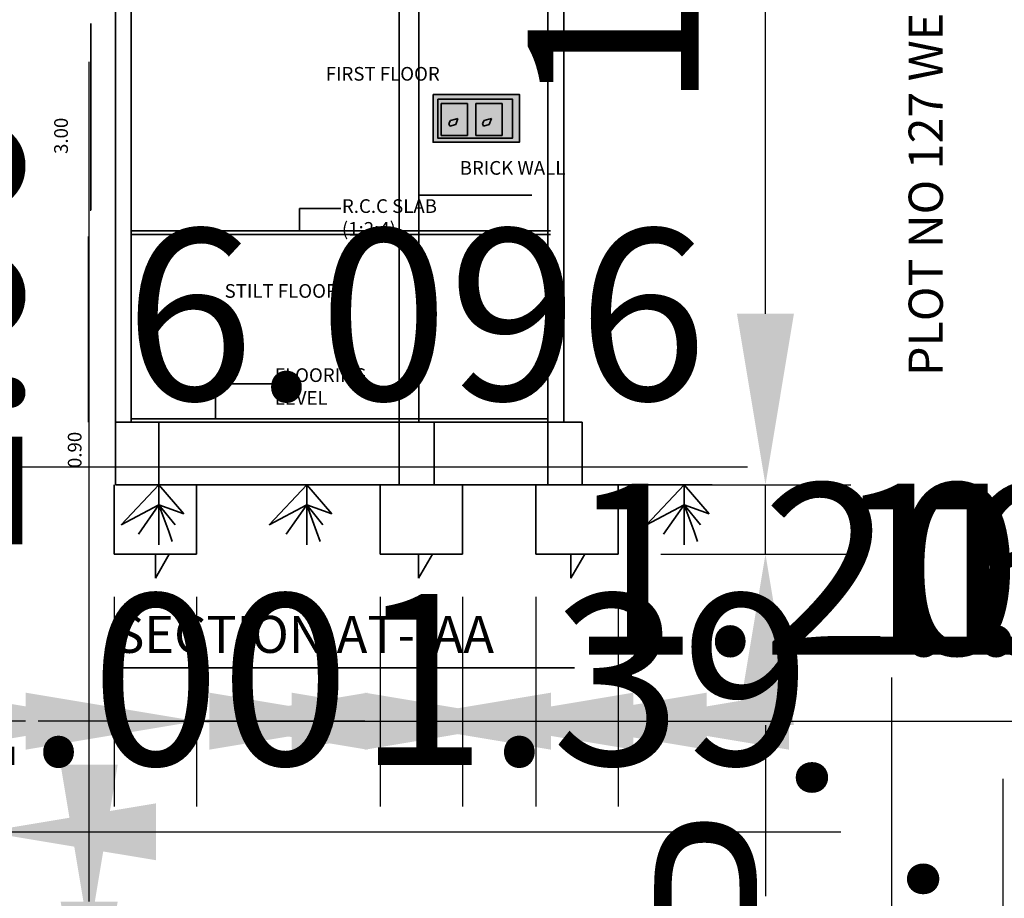
# Model space of a CAD drawing. Units: metres. Extents: x 782 to 1487, y 1262 to 7446.
# Tile 20 of 25: x 801.93 to 816.33, y 1313.5 to 1326.35. Entities that reach past the tile are written whole.
import ezdxf

# ---------------------------------------------------------------- set-up
doc = ezdxf.new("R2010")
doc.units = ezdxf.units.M
for name, color, linetype, lineweight in [('A-ANNO-DIMS', 2, 'Continuous', 18), ('A-ANNO-TEXT', 3, 'Continuous', 18), ('A-SECT', 7, 'Continuous', 35), ('A-SECT-PATT', 9, 'Continuous', 13)]:
    doc.layers.add(name, color=color, linetype=linetype, lineweight=lineweight)
doc.styles.get("Standard").update_dxf_attribs({"font": 'arial.ttf'})
doc.dimstyles.new('ISO-25', dxfattribs={"dimtxt": 2.5, "dimasz": 2.5, "dimexe": 1.25, "dimexo": 0.625, "dimtad": 1, "dimtxsty": 'Standard', "dimcen": 2.5, "dimadec": 0, "dimazin": 0, "dimtfac": 1, "dimtmove": 0, "dimatfit": 3, "dimfxl": 1, "dimarcsym": 0})

# ---------------------------------------------------------------- blocks, each defined once
blk = doc.blocks.new('*D2')
at = {"layer": 'A-ANNO-DIMS', "color": 0, "lineweight": -2, "transparency": 16777216}
for p, q in [((794.559, 1311.575), (794.559, 1314.2)), ((800.039, 1311.575), (800.039, 1314.2)), ((792.059, 1312.95), (781.81, 1312.95)), ((800.039, 1312.95), (794.559, 1312.95)), ((802.539, 1312.95), (805.039, 1312.95))]:
    blk.add_line(p, q, dxfattribs=at)
at = {"layer": 'A-ANNO-DIMS', "color": 0, "transparency": 16777216}
for points in [[(792.059, 1313.367), (792.059, 1312.534), (794.559, 1312.95)], [(802.539, 1313.367), (802.539, 1312.534), (800.039, 1312.95)]]:
    blk.add_solid(points, dxfattribs=at)
at = {"layer": 'Defpoints', "color": 0, "transparency": 16777216}
for p in [(794.559, 1312.95), (794.559, 1310.95), (800.039, 1310.95)]:
    blk.add_point(p, dxfattribs=at)
at = {"layer": 'A-ANNO-DIMS', "color": 0, "transparency": 16777216, "insert": (785.685, 1315.078), "char_height": 2.5, "width": 6.51678, "attachment_point": 5}
blk.add_mtext('5,48', dxfattribs=at)
blk = doc.blocks.new('*D23')
at = {"layer": 'A-ANNO-DIMS', "color": 0, "lineweight": -2, "transparency": 16777216}
for p, q in [((816.313, 1296.414), (816.313, 1315.246)), ((816.313, 1293.067), (816.313, 1293.914)), ((816.804, 1293.914), (817.563, 1293.914)), ((816.804, 1293.067), (817.563, 1293.067)), ((816.313, 1290.567), (816.313, 1288.067))]:
    blk.add_line(p, q, dxfattribs=at)
at = {"layer": 'A-ANNO-DIMS', "color": 0, "transparency": 16777216}
for points in [[(815.896, 1296.414), (816.729, 1296.414), (816.313, 1293.914)], [(815.896, 1290.567), (816.729, 1290.567), (816.313, 1293.067)]]:
    blk.add_solid(points, dxfattribs=at)
at = {"layer": 'Defpoints', "color": 0, "transparency": 16777216}
for p in [(816.179, 1293.914), (816.313, 1293.914), (816.179, 1293.067)]:
    blk.add_point(p, dxfattribs=at)
at = {"layer": 'A-ANNO-DIMS', "color": 0, "transparency": 16777216, "insert": (814.411, 1307.08), "char_height": 2.5, "attachment_point": 5, "rotation": 90}
blk.add_mtext('0.85 TYP.', dxfattribs=at)
blk = doc.blocks.new('*D25')
at = {"layer": 'A-ANNO-DIMS', "color": 0, "lineweight": -2, "transparency": 16777216}
for p, q in [((814.687, 1297.897), (814.687, 1316.729)), ((814.687, 1294.551), (814.687, 1295.397)), ((815.184, 1295.397), (815.937, 1295.397)), ((815.184, 1294.551), (815.937, 1294.551)), ((814.687, 1292.051), (814.687, 1289.551))]:
    blk.add_line(p, q, dxfattribs=at)
at = {"layer": 'A-ANNO-DIMS', "color": 0, "transparency": 16777216}
for points in [[(814.27, 1297.897), (815.103, 1297.897), (814.687, 1295.397)], [(814.27, 1292.051), (815.103, 1292.051), (814.687, 1294.551)]]:
    blk.add_solid(points, dxfattribs=at)
at = {"layer": 'Defpoints', "color": 0, "transparency": 16777216}
for p in [(814.559, 1295.397), (814.687, 1295.397), (814.559, 1294.551)]:
    blk.add_point(p, dxfattribs=at)
at = {"layer": 'A-ANNO-DIMS', "color": 0, "transparency": 16777216, "insert": (812.785, 1308.563), "char_height": 2.5, "attachment_point": 5, "rotation": 90}
blk.add_mtext('0.85 TYP.', dxfattribs=at)
blk = doc.blocks.new('*D37')
at = {"layer": 'A-ANNO-DIMS', "color": 0, "lineweight": -2, "transparency": 16777216}
for p, q in [((802.949, 1313.45), (802.949, 1315.95)), ((800.664, 1310.95), (804.199, 1310.95)), ((802.949, 1310.95), (802.949, 1307.03)), ((800.653, 1307.03), (804.199, 1307.03)), ((802.949, 1304.53), (802.949, 1294.314))]:
    blk.add_line(p, q, dxfattribs=at)
at = {"layer": 'A-ANNO-DIMS', "color": 0, "transparency": 16777216}
for points in [[(802.532, 1313.45), (803.366, 1313.45), (802.949, 1310.95)], [(802.532, 1304.53), (803.366, 1304.53), (802.949, 1307.03)]]:
    blk.add_solid(points, dxfattribs=at)
at = {"layer": 'Defpoints', "color": 0, "transparency": 16777216}
for p in [(800.039, 1310.95), (800.028, 1307.03), (802.949, 1307.03)]:
    blk.add_point(p, dxfattribs=at)
at = {"layer": 'A-ANNO-DIMS', "color": 0, "transparency": 16777216, "insert": (801.047, 1298.172), "char_height": 2.5, "attachment_point": 5, "rotation": 90}
blk.add_mtext('3.92', dxfattribs=at)
blk = doc.blocks.new('*D43')
at = {"layer": 'A-ANNO-DIMS', "color": 0, "lineweight": -2, "transparency": 16777216}
for p, q in [((792.559, 1313.575), (792.559, 1315.72)), ((794.559, 1311.575), (794.559, 1315.72)), ((790.059, 1314.47), (787.559, 1314.47)), ((792.559, 1314.47), (794.559, 1314.47)), ((797.059, 1314.47), (807.337, 1314.47))]:
    blk.add_line(p, q, dxfattribs=at)
at = {"layer": 'A-ANNO-DIMS', "color": 0, "transparency": 16777216}
for points in [[(790.059, 1314.887), (790.059, 1314.054), (792.559, 1314.47)], [(797.059, 1314.887), (797.059, 1314.054), (794.559, 1314.47)]]:
    blk.add_solid(points, dxfattribs=at)
at = {"layer": 'Defpoints', "color": 0, "transparency": 16777216}
for p in [(794.559, 1314.47), (792.559, 1312.95), (794.559, 1310.95)]:
    blk.add_point(p, dxfattribs=at)
at = {"layer": 'A-ANNO-DIMS', "color": 0, "transparency": 16777216, "insert": (803.448, 1316.372), "char_height": 2.5, "attachment_point": 5}
blk.add_mtext('2.00', dxfattribs=at)
blk = doc.blocks.new('*D44')
at = {"layer": 'A-ANNO-DIMS', "color": 0, "lineweight": -2, "transparency": 16777216}
for p, q in [((800.039, 1311.575), (800.039, 1315.72)), ((801.429, 1313.575), (801.429, 1315.72)), ((797.539, 1314.47), (795.039, 1314.47)), ((800.039, 1314.47), (801.429, 1314.47)), ((803.929, 1314.47), (813.943, 1314.47))]:
    blk.add_line(p, q, dxfattribs=at)
at = {"layer": 'A-ANNO-DIMS', "color": 0, "transparency": 16777216}
for points in [[(797.539, 1314.887), (797.539, 1314.054), (800.039, 1314.47)], [(803.929, 1314.887), (803.929, 1314.054), (801.429, 1314.47)]]:
    blk.add_solid(points, dxfattribs=at)
at = {"layer": 'Defpoints', "color": 0, "transparency": 16777216}
for p in [(801.429, 1314.47), (801.429, 1312.95), (800.039, 1310.95)]:
    blk.add_point(p, dxfattribs=at)
at = {"layer": 'A-ANNO-DIMS', "color": 0, "transparency": 16777216, "insert": (810.186, 1316.373), "char_height": 2.5, "attachment_point": 5}
blk.add_mtext('1.39', dxfattribs=at)
blk = doc.blocks.new('*D47')
at = {"layer": 'A-ANNO-DIMS', "color": 0, "lineweight": -2, "transparency": 16777216}
for p, q in [((802.949, 1315.45), (802.949, 1325.728)), ((802.054, 1312.95), (804.199, 1312.95)), ((802.949, 1310.95), (802.949, 1312.95)), ((800.664, 1310.95), (804.199, 1310.95)), ((802.949, 1308.45), (802.949, 1305.95))]:
    blk.add_line(p, q, dxfattribs=at)
at = {"layer": 'A-ANNO-DIMS', "color": 0, "transparency": 16777216}
for points in [[(802.532, 1315.45), (803.366, 1315.45), (802.949, 1312.95)], [(802.532, 1308.45), (803.366, 1308.45), (802.949, 1310.95)]]:
    blk.add_solid(points, dxfattribs=at)
at = {"layer": 'Defpoints', "color": 0, "transparency": 16777216}
for p in [(801.429, 1312.95), (802.949, 1312.95), (800.039, 1310.95)]:
    blk.add_point(p, dxfattribs=at)
at = {"layer": 'A-ANNO-DIMS', "color": 0, "transparency": 16777216, "insert": (801.048, 1321.839), "char_height": 2.5, "attachment_point": 5, "rotation": 90}
blk.add_mtext('2.00', dxfattribs=at)
blk = doc.blocks.new('*D115')
at = {"layer": 'A-ANNO-DIMS', "color": 0, "lineweight": -2, "transparency": 16777216}
for p, q in [((789.282, 1319.809), (786.782, 1319.809)), ((791.782, 1319.834), (791.782, 1318.559)), ((791.782, 1319.809), (797.878, 1319.809)), ((797.878, 1319.834), (797.878, 1318.559)), ((800.378, 1319.809), (812.576, 1319.809))]:
    blk.add_line(p, q, dxfattribs=at)
at = {"layer": 'A-ANNO-DIMS', "color": 0, "transparency": 16777216}
for points in [[(789.282, 1320.226), (789.282, 1319.392), (791.782, 1319.809)], [(800.378, 1320.226), (800.378, 1319.392), (797.878, 1319.809)]]:
    blk.add_solid(points, dxfattribs=at)
at = {"layer": 'Defpoints', "color": 0, "transparency": 16777216}
for p in [(791.782, 1320.459), (797.878, 1320.459), (797.878, 1319.809)]:
    blk.add_point(p, dxfattribs=at)
at = {"layer": 'A-ANNO-DIMS', "color": 0, "transparency": 16777216, "insert": (807.727, 1321.711), "char_height": 2.5, "attachment_point": 5}
blk.add_mtext('6.096', dxfattribs=at)
blk = doc.blocks.new('*D140')
at = {"layer": 'A-ANNO-DIMS', "color": 0, "lineweight": -2, "transparency": 16777216}
for p, q in [((803.316, 1317.905), (803.316, 1314.838)), ((804.52, 1317.905), (804.52, 1314.838)), ((800.816, 1316.088), (798.316, 1316.088)), ((803.316, 1316.088), (804.52, 1316.088)), ((807.02, 1316.088), (817.02, 1316.088))]:
    blk.add_line(p, q, dxfattribs=at)
at = {"layer": 'A-ANNO-DIMS', "color": 0, "transparency": 16777216}
for points in [[(800.816, 1316.505), (800.816, 1315.671), (803.316, 1316.088)], [(807.02, 1316.505), (807.02, 1315.671), (804.52, 1316.088)]]:
    blk.add_solid(points, dxfattribs=at)
at = {"layer": 'Defpoints', "color": 0, "transparency": 16777216}
for p in [(803.316, 1318.53), (804.52, 1318.53), (804.52, 1316.088)]:
    blk.add_point(p, dxfattribs=at)
at = {"layer": 'A-ANNO-DIMS', "color": 0, "transparency": 16777216, "insert": (813.27, 1317.989), "char_height": 2.5, "attachment_point": 5}
blk.add_mtext('1.20', dxfattribs=at)
blk = doc.blocks.new('*D141')
at = {"layer": 'A-ANNO-DIMS', "color": 0, "lineweight": -2, "transparency": 16777216}
for p, q in [((804.52, 1317.905), (804.52, 1314.838)), ((807.205, 1317.905), (807.205, 1314.838)), ((802.02, 1316.088), (799.52, 1316.088)), ((804.52, 1316.088), (807.205, 1316.088)), ((809.705, 1316.088), (819.997, 1316.088))]:
    blk.add_line(p, q, dxfattribs=at)
at = {"layer": 'A-ANNO-DIMS', "color": 0, "transparency": 16777216}
for points in [[(802.02, 1316.505), (802.02, 1315.671), (804.52, 1316.088)], [(809.705, 1316.505), (809.705, 1315.671), (807.205, 1316.088)]]:
    blk.add_solid(points, dxfattribs=at)
at = {"layer": 'Defpoints', "color": 0, "transparency": 16777216}
for p in [(804.52, 1318.53), (807.205, 1318.53), (807.205, 1316.088)]:
    blk.add_point(p, dxfattribs=at)
at = {"layer": 'A-ANNO-DIMS', "color": 0, "transparency": 16777216, "insert": (816.101, 1317.989), "char_height": 2.5, "attachment_point": 5}
blk.add_mtext('2.68', dxfattribs=at)
blk = doc.blocks.new('*D142')
at = {"layer": 'A-ANNO-DIMS', "color": 0, "lineweight": -2, "transparency": 16777216}
for p, q in [((807.205, 1317.905), (807.205, 1314.838)), ((808.409, 1317.905), (808.409, 1314.838)), ((804.705, 1316.088), (802.205, 1316.088)), ((807.205, 1316.088), (808.409, 1316.088)), ((810.909, 1316.088), (820.909, 1316.088))]:
    blk.add_line(p, q, dxfattribs=at)
at = {"layer": 'A-ANNO-DIMS', "color": 0, "transparency": 16777216}
for points in [[(804.705, 1316.505), (804.705, 1315.671), (807.205, 1316.088)], [(810.909, 1316.505), (810.909, 1315.671), (808.409, 1316.088)]]:
    blk.add_solid(points, dxfattribs=at)
at = {"layer": 'Defpoints', "color": 0, "transparency": 16777216}
for p in [(807.205, 1318.53), (808.409, 1318.53), (808.409, 1316.088)]:
    blk.add_point(p, dxfattribs=at)
at = {"layer": 'A-ANNO-DIMS', "color": 0, "transparency": 16777216, "insert": (817.159, 1317.989), "char_height": 2.5, "attachment_point": 5}
blk.add_mtext('1.20', dxfattribs=at)
blk = doc.blocks.new('*D143')
at = {"layer": 'A-ANNO-DIMS', "color": 0, "lineweight": -2, "transparency": 16777216}
for p, q in [((808.409, 1317.905), (808.409, 1314.838)), ((809.479, 1317.905), (809.479, 1314.838)), ((805.909, 1316.088), (803.409, 1316.088)), ((808.409, 1316.088), (809.479, 1316.088)), ((811.979, 1316.088), (821.987, 1316.088))]:
    blk.add_line(p, q, dxfattribs=at)
at = {"layer": 'A-ANNO-DIMS', "color": 0, "transparency": 16777216}
for points in [[(805.909, 1316.505), (805.909, 1315.671), (808.409, 1316.088)], [(811.979, 1316.505), (811.979, 1315.671), (809.479, 1316.088)]]:
    blk.add_solid(points, dxfattribs=at)
at = {"layer": 'Defpoints', "color": 0, "transparency": 16777216}
for p in [(808.409, 1318.53), (809.479, 1318.53), (809.479, 1316.088)]:
    blk.add_point(p, dxfattribs=at)
at = {"layer": 'A-ANNO-DIMS', "color": 0, "transparency": 16777216, "insert": (818.233, 1317.989), "char_height": 2.5, "attachment_point": 5}
blk.add_mtext('1.07', dxfattribs=at)
blk = doc.blocks.new('*D144')
at = {"layer": 'A-ANNO-DIMS', "color": 0, "lineweight": -2, "transparency": 16777216}
for p, q in [((809.479, 1317.905), (809.479, 1314.838)), ((810.683, 1317.905), (810.683, 1314.838)), ((806.979, 1316.088), (804.479, 1316.088)), ((809.479, 1316.088), (810.683, 1316.088)), ((813.183, 1316.088), (823.183, 1316.088))]:
    blk.add_line(p, q, dxfattribs=at)
at = {"layer": 'A-ANNO-DIMS', "color": 0, "transparency": 16777216}
for points in [[(806.979, 1316.505), (806.979, 1315.671), (809.479, 1316.088)], [(813.183, 1316.505), (813.183, 1315.671), (810.683, 1316.088)]]:
    blk.add_solid(points, dxfattribs=at)
at = {"layer": 'Defpoints', "color": 0, "transparency": 16777216}
for p in [(809.479, 1318.53), (810.683, 1318.53), (810.683, 1316.088)]:
    blk.add_point(p, dxfattribs=at)
at = {"layer": 'A-ANNO-DIMS', "color": 0, "transparency": 16777216, "insert": (819.433, 1317.989), "char_height": 2.5, "attachment_point": 5}
blk.add_mtext('1.20', dxfattribs=at)
blk = doc.blocks.new('*D145')
at = {"layer": 'A-ANNO-DIMS', "color": 0, "lineweight": -2, "transparency": 16777216}
for p, q in [((812.839, 1322.045), (812.839, 1334.015)), ((811.308, 1319.545), (814.089, 1319.545)), ((812.839, 1318.53), (812.839, 1319.545)), ((811.308, 1318.53), (814.089, 1318.53)), ((812.839, 1316.03), (812.839, 1313.53))]:
    blk.add_line(p, q, dxfattribs=at)
at = {"layer": 'A-ANNO-DIMS', "color": 0, "transparency": 16777216}
for points in [[(812.422, 1322.045), (813.255, 1322.045), (812.839, 1319.545)], [(812.422, 1316.03), (813.255, 1316.03), (812.839, 1318.53)]]:
    blk.add_solid(points, dxfattribs=at)
at = {"layer": 'Defpoints', "color": 0, "transparency": 16777216}
for p in [(810.683, 1319.545), (812.839, 1319.545), (810.683, 1318.53)]:
    blk.add_point(p, dxfattribs=at)
at = {"layer": 'A-ANNO-DIMS', "color": 0, "transparency": 16777216, "insert": (810.937, 1329.28), "char_height": 2.5, "attachment_point": 5, "rotation": 90}
blk.add_mtext('1.015', dxfattribs=at)
blk = doc.blocks.new('*D146')
at = {"layer": 'A-ANNO-DIMS', "color": 0, "lineweight": -2, "transparency": 16777216}
for p, q in [((812.839, 1330.363), (812.839, 1344.262)), ((810.513, 1330.363), (814.089, 1330.363)), ((812.839, 1322.045), (812.839, 1327.863)), ((810.513, 1319.545), (814.089, 1319.545))]:
    blk.add_line(p, q, dxfattribs=at)
at = {"layer": 'A-ANNO-DIMS', "color": 0, "transparency": 16777216}
for points in [[(812.422, 1327.863), (813.255, 1327.863), (812.839, 1330.363)], [(812.422, 1322.045), (813.255, 1322.045), (812.839, 1319.545)]]:
    blk.add_solid(points, dxfattribs=at)
at = {"layer": 'Defpoints', "color": 0, "transparency": 16777216}
for p in [(809.888, 1330.363), (812.839, 1330.363), (809.888, 1319.545)]:
    blk.add_point(p, dxfattribs=at)
at = {"layer": 'A-ANNO-DIMS', "color": 0, "transparency": 16777216, "insert": (810.937, 1338.563), "char_height": 2.5, "attachment_point": 5, "rotation": 90}
blk.add_mtext('10.818', dxfattribs=at)

msp = doc.modelspace()

# ---------------------------------------------------------------- hatches: boundary and pattern name
at = {"layer": 'A-SECT-PATT'}
h = msp.add_hatch(color=256, dxfattribs=at)
h.dxf.hatch_style = 1
h.paths.add_polyline_path([(809.2411, 1325.2532), (807.9777, 1325.2532), (807.9777, 1324.5546), (809.2411, 1324.5546)])
h.paths.add_polyline_path([(809.1376, 1324.6125), (808.0486, 1324.6125), (808.0486, 1325.1844), (809.1376, 1325.1844)], flags=16)
h.paths.add_polyline_path([(808.9875, 1324.6538), (808.6043, 1324.6538), (808.6043, 1325.1207), (808.9875, 1325.1207)], flags=0)
h.paths.add_polyline_path([(808.4803, 1324.6538), (808.0971, 1324.6538), (808.0971, 1325.1207), (808.4803, 1325.1207)], flags=0)
h = msp.add_hatch(color=256, dxfattribs=at)
h.dxf.hatch_style = 1
h.paths.add_polyline_path([(809.1376, 1325.1844), (808.0486, 1325.1844), (808.0486, 1324.6125), (809.1376, 1324.6125)])
h.paths.add_polyline_path([(808.4803, 1325.1207), (808.4803, 1324.6538), (808.0971, 1324.6538), (808.0971, 1325.1207)], flags=16)
h.paths.add_polyline_path([(808.3426, 1324.9005), (808.3106, 1324.8132), (808.224, 1324.7916), (808.2108, 1324.8301), (808.2343, 1324.8706), (808.3059, 1324.8903)], flags=0)
h.paths.add_polyline_path([(808.6043, 1325.1207), (808.9875, 1325.1207), (808.9875, 1324.6538), (808.6043, 1324.6538)], flags=16)
h.paths.add_polyline_path([(808.7238, 1324.8706), (808.7953, 1324.8903), (808.8321, 1324.9005), (808.8, 1324.8132), (808.7134, 1324.7916), (808.7002, 1324.8301)], flags=0)
h = msp.add_hatch(color=256, dxfattribs=at)
h.dxf.hatch_style = 1
h.paths.add_polyline_path([(808.4803, 1325.1207), (808.0971, 1325.1207), (808.0971, 1324.6538), (808.4803, 1324.6538)])
h.paths.add_polyline_path([(808.3106, 1324.8132), (808.224, 1324.7916), (808.2108, 1324.8301), (808.2343, 1324.8706), (808.3059, 1324.8903), (808.3426, 1324.9005)], flags=16)
h.paths.add_polyline_path([(808.9875, 1325.1207), (808.6043, 1325.1207), (808.6043, 1324.6538), (808.9875, 1324.6538)])
h.paths.add_polyline_path([(808.7238, 1324.8706), (808.7953, 1324.8903), (808.8321, 1324.9005), (808.8, 1324.8132), (808.7134, 1324.7916), (808.7002, 1324.8301)], flags=16)
h = msp.add_hatch(color=256, dxfattribs=at)
h.dxf.hatch_style = 1
h.paths.add_polyline_path([(808.3426, 1324.9005), (808.3059, 1324.8903), (808.2343, 1324.8706), (808.2108, 1324.8301), (808.224, 1324.7916), (808.3106, 1324.8132)])
h.paths.add_polyline_path([(808.8321, 1324.9005), (808.7953, 1324.8903), (808.7238, 1324.8706), (808.7002, 1324.8301), (808.7134, 1324.7916), (808.8, 1324.8132)])

# ---------------------------------------------------------------- linework, layer by layer
at = {"layer": 'A-SECT'}
for p, q in [((803.3321, 1320.4591), (803.3321, 1330.3635)), ((803.5621, 1320.4591), (803.5621, 1330.3635)), ((809.6581, 1320.4591), (809.6581, 1330.3635)), ((809.8881, 1320.4591), (809.8881, 1330.3635)), ((807.4812, 1320.4591), (807.4812, 1329.4495)), ((807.7695, 1320.4591), (807.7695, 1329.4495)), ((802.9742, 1323.5616), (802.9742, 1326.2912)), ((803.5621, 1325.4113), (803.5621, 1324.2292)), ((807.7695, 1324.9543), (807.7695, 1323.7795)), ((808.2108, 1324.8301), (808.2343, 1324.8706)), ((808.224, 1324.7916), (808.2108, 1324.8301)), ((808.3106, 1324.8132), (808.224, 1324.7916)), ((808.2343, 1324.8706), (808.3059, 1324.8903)), ((808.3059, 1324.8903), (808.3426, 1324.9005)), ((808.3426, 1324.9005), (808.3106, 1324.8132)), ((808.7002, 1324.8301), (808.7238, 1324.8706)), ((808.7134, 1324.7916), (808.7002, 1324.8301)), ((808.8, 1324.8132), (808.7134, 1324.7916)), ((808.7238, 1324.8706), (808.7953, 1324.8903)), ((808.7953, 1324.8903), (808.8321, 1324.9005)), ((808.8321, 1324.9005), (808.8, 1324.8132)), ((807.7695, 1323.7795), (809.4239, 1323.7795)), ((802.9645, 1323.5616), (802.9742, 1323.5616)), ((806.0261, 1323.257), (806.0261, 1323.5868)), ((806.0261, 1323.5868), (806.6295, 1323.5868)), ((803.5621, 1323.257), (809.6969, 1323.257)), ((803.5621, 1323.2062), (809.6969, 1323.2062)), ((806.6295, 1323.257), (806.0261, 1323.257)), ((802.9415, 1320.4591), (802.9415, 1323.1735)), ((804.7975, 1320.5099), (804.7975, 1321.0213)), ((804.7975, 1321.0213), (805.6623, 1321.0213)), ((803.5621, 1320.4591), (803.3321, 1320.4591)), ((803.5621, 1320.4591), (803.3321, 1320.4591)), ((803.3321, 1320.4591), (803.3321, 1319.5451)), ((803.5621, 1320.5099), (809.6581, 1320.5099)), ((803.5621, 1320.5099), (803.5621, 1320.4591)), ((803.5621, 1320.5099), (804.7975, 1320.5099)), ((803.5621, 1320.4591), (809.6581, 1320.4591)), ((803.97, 1319.5451), (803.97, 1320.4591)), ((807.9953, 1320.4591), (807.3522, 1320.4591)), ((807.4812, 1320.5099), (807.4812, 1319.5451)), ((807.9953, 1319.5451), (807.9953, 1320.4591)), ((809.6581, 1319.5451), (809.6581, 1320.4591)), ((809.8881, 1320.4591), (809.6581, 1320.4591)), ((809.6581, 1320.4591), (809.8881, 1320.4591)), ((809.8881, 1320.4591), (810.1568, 1320.4591)), ((810.1568, 1320.4591), (810.1568, 1319.5552)), ((803.3164, 1318.53), (803.3164, 1319.5451)), ((803.3321, 1319.5451), (803.5621, 1319.5451)), ((803.4195, 1318.9602), (803.97, 1319.5451)), ((803.5621, 1319.5451), (809.6581, 1319.5451)), ((803.5621, 1319.5451), (803.97, 1319.5451)), ((803.97, 1319.5451), (803.97, 1318.6681)), ((803.97, 1318.6681), (803.97, 1319.5451)), ((803.97, 1319.5451), (803.97, 1319.2527)), ((803.97, 1319.5451), (804.3358, 1319.1194)), ((804.5202, 1319.5451), (804.5202, 1318.53)), ((805.5817, 1318.9602), (806.1321, 1319.5451)), ((806.1321, 1319.5451), (806.1321, 1318.6681)), ((806.1321, 1318.6681), (806.1321, 1319.5451)), ((806.1321, 1319.5451), (806.1321, 1319.2527)), ((806.1321, 1319.5451), (806.4979, 1319.1194)), ((807.205, 1318.53), (807.205, 1319.5451)), ((807.4812, 1319.5451), (807.9953, 1319.5451)), ((808.4088, 1319.5451), (808.4088, 1318.53)), ((809.4788, 1318.53), (809.4788, 1319.5451)), ((809.8881, 1319.5451), (809.6581, 1319.5451)), ((809.6581, 1319.5451), (809.8881, 1319.5451)), ((810.1568, 1319.5451), (809.8881, 1319.5451)), ((810.1568, 1319.5552), (810.1568, 1319.5451)), ((810.1568, 1319.5451), (810.6826, 1319.5451)), ((810.6826, 1319.5451), (812.0587, 1319.5451)), ((811.1013, 1318.9602), (811.6517, 1319.5451)), ((811.6517, 1319.5451), (811.6517, 1318.6681)), ((811.6517, 1318.6681), (811.6517, 1319.5451)), ((811.6517, 1319.5451), (811.6517, 1319.2527)), ((811.6517, 1319.5451), (812.0175, 1319.1194)), ((803.97, 1319.2527), (803.4195, 1318.9602)), ((803.97, 1319.2527), (803.4195, 1318.9602)), ((803.97, 1319.2527), (803.6685, 1318.8209)), ((804.3358, 1319.1194), (803.97, 1319.2527)), ((803.97, 1319.2527), (804.2063, 1318.9602)), ((803.97, 1319.2527), (804.1122, 1318.8615)), ((806.1321, 1319.2527), (805.5817, 1318.9602)), ((806.1321, 1319.2527), (805.5817, 1318.9602)), ((806.1321, 1319.2527), (805.8306, 1318.8209)), ((806.4979, 1319.1194), (806.1321, 1319.2527)), ((806.1321, 1319.2527), (806.3685, 1318.9602)), ((806.1321, 1319.2527), (806.2744, 1318.8615)), ((811.6517, 1319.2527), (811.1013, 1318.9602)), ((811.6517, 1319.2527), (811.1013, 1318.9602)), ((811.6517, 1319.2527), (811.3502, 1318.8209)), ((812.0175, 1319.1194), (811.6517, 1319.2527)), ((811.6517, 1319.2527), (811.8881, 1318.9602)), ((811.6517, 1319.2527), (811.794, 1318.8615)), ((804.1122, 1318.8615), (804.1654, 1318.7154)), ((806.2744, 1318.8615), (806.3275, 1318.7154)), ((811.794, 1318.8615), (811.8471, 1318.7154)), ((804.5202, 1318.53), (803.3164, 1318.53)), ((803.9183, 1318.53), (803.9183, 1318.1785)), ((803.9183, 1318.1785), (803.9183, 1318.53)), ((803.9183, 1318.53), (804.12, 1318.53)), ((804.12, 1318.53), (803.9183, 1318.1785)), ((808.4088, 1318.53), (807.205, 1318.53)), ((807.7662, 1318.53), (807.7662, 1318.1785)), ((807.7662, 1318.1785), (807.7662, 1318.53)), ((807.9679, 1318.53), (807.7662, 1318.1785)), ((810.6826, 1318.53), (809.4788, 1318.53)), ((809.9944, 1318.53), (809.9944, 1318.1785)), ((809.9944, 1318.1785), (809.9944, 1318.53)), ((810.1961, 1318.53), (809.9944, 1318.1785)), ((803.2515, 1316.868), (810.0445, 1316.868))]:
    msp.add_line(p, q, dxfattribs=at)
for points in [[(807.9777, 1325.2532), (809.2411, 1325.2532), (809.2411, 1324.5546), (807.9777, 1324.5546)], [(808.0486, 1325.1844), (809.1376, 1325.1844), (809.1376, 1324.6125), (808.0486, 1324.6125)], [(808.0971, 1325.1207), (808.4803, 1325.1207), (808.4803, 1324.6538), (808.0971, 1324.6538)], [(808.6043, 1325.1207), (808.9875, 1325.1207), (808.9875, 1324.6538), (808.6043, 1324.6538)]]:
    msp.add_lwpolyline(points, close=True, dxfattribs=at)
msp.add_lwpolyline([(810.6826, 1319.5451), (810.6826, 1318.53)], dxfattribs=at)

# ---------------------------------------------------------------- texts
at = {"layer": 'A-ANNO-TEXT', "attachment_point": 1, "rotation": 90}
for s, width, insert, char_height in [('PLOT NO 127 WESTERN PART', 13.280177, (814.9325, 1321.1357), 0.5), ('\\P3.00', 0.796716, (802.1044, 1324.3824), 0.2), ('\\P0.90', 0.796716, (802.304, 1319.7897), 0.2)]:
    msp.add_mtext_dynamic_manual_height_columns(s, width=width, gutter_width=12.5, heights=[0], dxfattribs=dict(at, insert=insert, char_height=char_height))
at = {"layer": 'A-ANNO-TEXT', "attachment_point": 1}
for s, width, gutter_width, insert, char_height in [('\\PFIRST FLOOR', 3.249799, 12.5, (806.4083, 1325.9883), 0.2), ('\\PBRICK WALL', 1.630226, 12.5, (808.3676, 1324.6125), 0.2), ('\\PR.C.C SLAB (1:2:4)', 1.65154, 12.5, (806.6452, 1324.0538), 0.2), ('\\PSTILT FLOOR', 3.01159, 12.5, (804.9298, 1322.8129), 0.2), ('\\PFLOORING LEVEL', 2.004867, 12.5, (805.6623, 1321.5819), 0.2), ('\\PSECTION AT--AA', 26.571724, 33.8216, (803.3164, 1318.53), 0.541146)]:
    msp.add_mtext_dynamic_manual_height_columns(s, width=width, gutter_width=gutter_width, heights=[0], dxfattribs=dict(at, insert=insert, char_height=char_height))

# ---------------------------------------------------------------- dimensions: what is measured, and where the dimension line sits
at = {"layer": 'A-ANNO-DIMS'}
for base, p1, p2, override, picture, middle in [((812.8387, 1330.3635), (809.8881, 1319.5451), (809.8881, 1330.3635), {"dimdec": 3, "dimlfac": 1, "dimrnd": 0, "dimzin": 0, "dimdsep": 46, "dimlunit": 2}, '*D146', (810.9373, 1338.5627)), ((812.8387, 1319.5451), (810.6826, 1318.53), (810.6826, 1319.5451), {"dimdec": 3, "dimlfac": 1, "dimrnd": 0, "dimzin": 0, "dimdsep": 46, "dimlunit": 2}, '*D145', (810.9373, 1329.2799)), ((802.949, 1312.9503), (800.039, 1310.9503), (801.429, 1312.9503), {"dimdec": 2, "dimlfac": 1, "dimrnd": 0, "dimzin": 0, "dimdsep": 46, "dimlunit": 2}, '*D47', (801.0476, 1321.8393)), ((802.949, 1307.0305), (800.039, 1310.9503), (800.0278, 1307.0305), {"dimdec": 2, "dimlfac": 1, "dimrnd": 0, "dimzin": 0, "dimdsep": 46, "dimlunit": 2}, '*D37', (801.0468, 1298.1722))]:
    dim = msp.add_linear_dim(base=base, p1=p1, p2=p2, angle=90, dimstyle='ISO-25', override=override, dxfattribs=at)
    dim.commit()
    dim.dimension.update_dxf_attribs({"geometry": picture, "text_midpoint": middle})
for base, p1, p2, override, picture, middle in [((797.8778, 1319.8091), (791.7818, 1320.4591), (797.8778, 1320.4591), {"dimdec": 3, "dimlfac": 1, "dimrnd": 0, "dimzin": 0, "dimdsep": 46, "dimlunit": 2}, '*D115', (807.7269, 1321.7105)), ((804.5202, 1316.088), (803.3164, 1318.53), (804.5202, 1318.53), {"dimdec": 2, "dimlfac": 1, "dimrnd": 0, "dimzin": 0, "dimdsep": 46, "dimlunit": 2}, '*D140', (813.2702, 1317.9895)), ((807.205, 1316.088), (804.5202, 1318.53), (807.205, 1318.53), {"dimdec": 2, "dimlfac": 1, "dimrnd": 0, "dimzin": 0, "dimdsep": 46, "dimlunit": 2}, '*D141', (816.1008, 1317.9895)), ((808.4088, 1316.088), (807.205, 1318.53), (808.4088, 1318.53), {"dimdec": 2, "dimlfac": 1, "dimrnd": 0, "dimzin": 0, "dimdsep": 46, "dimlunit": 2}, '*D142', (817.1588, 1317.9895)), ((809.4788, 1316.088), (808.4088, 1318.53), (809.4788, 1318.53), {"dimdec": 2, "dimlfac": 1, "dimrnd": 0, "dimzin": 0, "dimdsep": 46, "dimlunit": 2}, '*D143', (818.2331, 1317.9895)), ((810.6826, 1316.088), (809.4788, 1318.53), (810.6826, 1318.53), {"dimdec": 2, "dimlfac": 1, "dimrnd": 0, "dimzin": 0, "dimdsep": 46, "dimlunit": 2}, '*D144', (819.4326, 1317.9895)), ((794.559, 1314.4703), (792.559, 1312.9503), (794.559, 1310.9503), {"dimdec": 2, "dimlfac": 1, "dimrnd": 0, "dimzin": 0, "dimdsep": 46, "dimlunit": 2}, '*D43', (803.448, 1316.3718)), ((801.429, 1314.4703), (800.039, 1310.9503), (801.429, 1312.9503), {"dimdec": 2, "dimlfac": 1, "dimrnd": 0, "dimzin": 0, "dimdsep": 46, "dimlunit": 2}, '*D44', (810.1859, 1316.3726)), ((794.559, 1312.9503), (800.039, 1310.9503), (794.559, 1310.9503), {"dimclrd": 0, "dimclre": 0, "dimclrt": 0}, '*D2', (785.6846, 1315.0777))]:
    dim = msp.add_linear_dim(base=base, p1=p1, p2=p2, dimstyle='ISO-25', override=override, dxfattribs=at)
    dim.commit()
    dim.dimension.update_dxf_attribs({"geometry": picture, "text_midpoint": middle})
for base, p1, p2, picture, middle in [((814.6868, 1295.3974), (814.5592, 1294.5507), (814.5592, 1295.3974), '*D25', (812.7854, 1308.5633)), ((816.3126, 1293.9141), (816.1792, 1293.0674), (816.1792, 1293.9141), '*D23', (814.4112, 1307.08))]:
    dim = msp.add_linear_dim(base=base, p1=p1, p2=p2, angle=90, text='<> TYP.', dimstyle='ISO-25', override={"dimdec": 2, "dimlfac": 1, "dimrnd": 0, "dimzin": 0, "dimdsep": 46, "dimlunit": 2}, dxfattribs=at)
    dim.commit()
    dim.dimension.update_dxf_attribs({"geometry": picture, "text_midpoint": middle})

doc.saveas('drawing.dxf')
